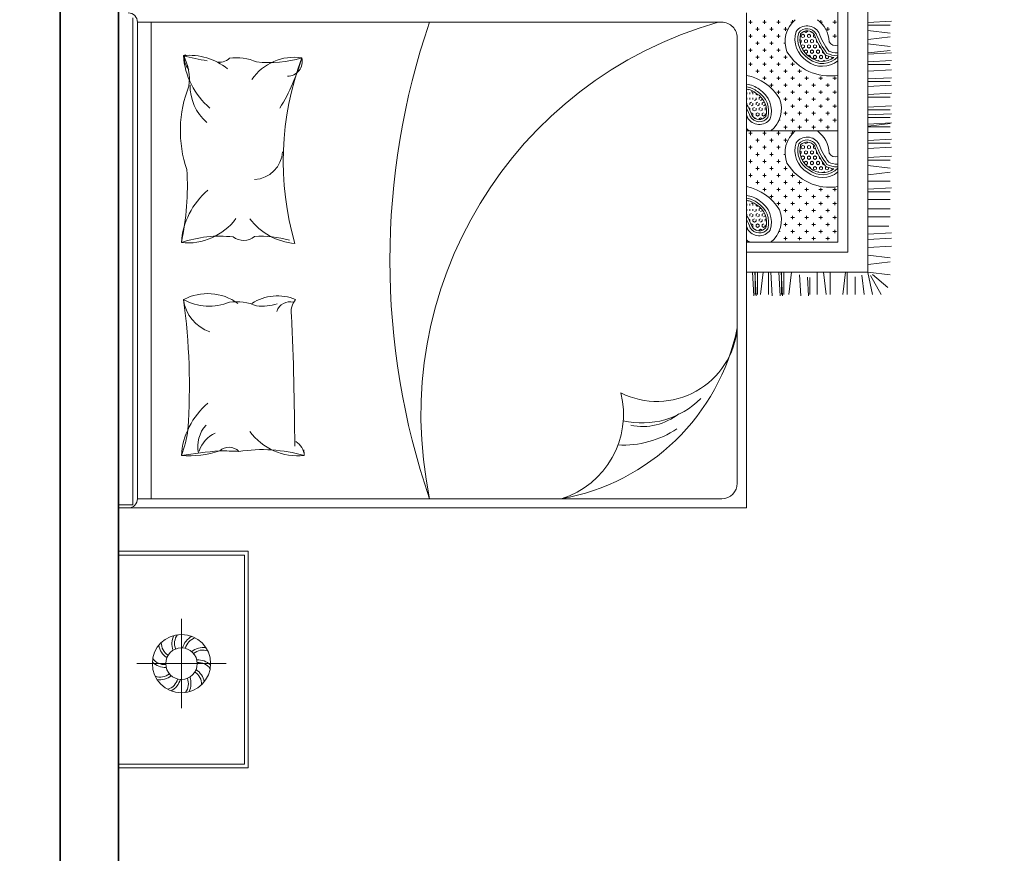
# Model space of a CAD drawing. Units: inches. Extents: x -638 to 186, y -762 to 59.
# Tile 16 of 31: x -168 to -92, y -308 to -243. Entities that reach past the tile are written whole.
import ezdxf

# ---------------------------------------------------------------- set-up
doc = ezdxf.new("R2010")
doc.units = ezdxf.units.IN
for name, color, linetype, lineweight in [('A-ANNO-DIMS', 2, 'Continuous', 18), ('furn', 8, 'Continuous', 13), ('wall', 7, 'Continuous', 35)]:
    doc.layers.add(name, color=color, linetype=linetype, lineweight=lineweight)
doc.styles.get("Standard").update_dxf_attribs({"font": 'arial.ttf'})
doc.dimstyles.new('ISO-25', dxfattribs={"dimtxt": 4, "dimasz": 4, "dimexe": 1.25, "dimexo": 0.625, "dimtad": 0, "dimlunit": 4, "dimtxsty": 'Standard', "dimcen": 2.5, "dimclrt": 256, "dimadec": 0, "dimazin": 0, "dimtfac": 1, "dimtmove": 0, "dimatfit": 3, "dimfxl": 1, "dimfxlon": 1, "dimarcsym": 0})

# ---------------------------------------------------------------- blocks, each defined once
blk = doc.blocks.new('BED-DOUBLE-WITH-NIGHTSTANDS')
for p, q in [((0, 59.951), (78.699, 59.951)), ((0, 49.874), (0, 59.951)), ((0.288, 50.162), (0.288, 59.951)), ((16.508, 59.951), (16.508, 50.162)), ((16.796, 59.951), (16.796, 49.874)), ((20.158, 59.951), (20.158, 11.244)), ((20.398, 58.826), (20.398, 59.951)), ((58.161, 58.826), (20.398, 58.826)), ((8.091, 51.596), (8.091, 58.516)), ((20.878, 58.468), (57.828, 58.468)), ((20.878, 58.468), (20.878, 13.164)), ((57.828, 13.164), (57.828, 58.468)), ((57.828, 57.404), (20.878, 57.404)), ((4.631, 55.056), (11.551, 55.056)), ((16.796, 49.874), (0, 49.874)), ((16.508, 50.162), (0.288, 50.162)), ((22.077, 11.964), (56.628, 11.964)), ((20.158, 11.244), (58.548, 11.244)), ((38.435, 10.789), (36.606, 10.687)), ((38.435, 1.829), (38.435, 11.244)), ((39.99, 3.384), (39.99, 11.244)), ((40.767, 4.161), (40.767, 11.244)), ((41.943, 10.806), (41.98, 10.743)), ((42.116, 10.743), (41.98, 10.743)), ((42.184, 10.861), (42.116, 10.743)), ((42.164, 10.895), (42.184, 10.861)), ((42.388, 10.743), (42.32, 10.625)), ((42.381, 10.99), (42.388, 10.979)), ((42.524, 10.979), (42.388, 10.979)), ((42.524, 10.743), (42.388, 10.743)), ((42.588, 11.09), (42.524, 10.979)), ((42.524, 10.743), (42.592, 10.625)), ((42.728, 10.861), (42.796, 10.743)), ((42.932, 10.979), (42.796, 10.979)), ((42.932, 10.743), (42.796, 10.743)), ((42.932, 11.215), (42.819, 11.215)), ((42.932, 10.979), (43, 10.861)), ((43.34, 11.215), (43.204, 11.215)), ((43.34, 10.979), (43.204, 10.979)), ((43.34, 10.743), (43.204, 10.743)), ((43.748, 11.215), (43.612, 11.215)), ((43.748, 10.979), (43.612, 10.979)), ((43.748, 10.743), (43.612, 10.743)), ((43.816, 10.861), (43.748, 10.743)), ((44.002, 11.184), (43.952, 11.097)), ((45.812, 10.936), (46.084, 10.936)), ((45.948, 10.8), (45.948, 11.072)), ((46.9, 10.936), (47.172, 10.936)), ((47.036, 10.8), (47.036, 11.072)), ((47.989, 10.936), (48.261, 10.936)), ((48.125, 10.8), (48.125, 11.072)), ((49.077, 10.936), (49.349, 10.936)), ((49.213, 10.8), (49.213, 11.072)), ((49.395, 11.244), (49.395, 4.161)), ((50.571, 10.806), (50.607, 10.743)), ((50.743, 10.743), (50.607, 10.743)), ((50.811, 10.861), (50.743, 10.743)), ((50.792, 10.895), (50.811, 10.861)), ((51.015, 10.743), (50.947, 10.625)), ((51.009, 10.99), (51.015, 10.979)), ((51.151, 10.979), (51.015, 10.979)), ((51.151, 10.743), (51.015, 10.743)), ((51.216, 11.09), (51.151, 10.979)), ((51.151, 10.743), (51.219, 10.625)), ((51.355, 10.861), (51.424, 10.743)), ((51.56, 10.979), (51.424, 10.979)), ((51.56, 10.743), (51.424, 10.743)), ((51.56, 11.215), (51.447, 11.215)), ((51.56, 10.979), (51.628, 10.861)), ((51.968, 11.215), (51.832, 11.215)), ((51.968, 10.979), (51.832, 10.979)), ((51.968, 10.743), (51.832, 10.743)), ((52.376, 11.215), (52.24, 11.215)), ((52.376, 10.979), (52.24, 10.979)), ((52.376, 10.743), (52.24, 10.743)), ((52.444, 10.861), (52.376, 10.743)), ((52.63, 11.184), (52.58, 11.097)), ((54.44, 10.936), (54.712, 10.936)), ((54.576, 10.8), (54.576, 11.072)), ((55.528, 10.936), (55.8, 10.936)), ((55.664, 10.8), (55.664, 11.072)), ((56.616, 10.936), (56.888, 10.936)), ((56.752, 10.8), (56.752, 11.072)), ((57.705, 10.936), (57.977, 10.936)), ((57.841, 10.8), (57.841, 11.072)), ((38.435, 10.606), (36.606, 10.504)), ((38.435, 10.585), (36.707, 10.585)), ((38.435, 10.402), (36.707, 10.402)), ((38.435, 9.957), (36.707, 10.161)), ((41.708, 10.272), (41.649, 10.272)), ((41.708, 10.036), (41.685, 10.036)), ((41.708, 10.508), (41.699, 10.508)), ((41.776, 10.625), (41.708, 10.508)), ((41.708, 10.272), (41.776, 10.154)), ((41.776, 10.154), (41.708, 10.036)), ((41.77, 10.636), (41.776, 10.625)), ((41.98, 10.508), (41.912, 10.39)), ((41.912, 10.39), (41.98, 10.272)), ((41.98, 10.036), (41.912, 9.919)), ((42.116, 10.508), (41.98, 10.508)), ((42.116, 10.272), (41.98, 10.272)), ((42.116, 10.036), (41.98, 10.036)), ((42.116, 10.508), (42.184, 10.39)), ((42.184, 10.39), (42.116, 10.272)), ((42.116, 10.036), (42.184, 9.919)), ((42.32, 10.625), (42.388, 10.508)), ((42.32, 10.154), (42.388, 10.036)), ((42.524, 10.508), (42.388, 10.508)), ((42.524, 10.272), (42.388, 10.272)), ((42.524, 10.036), (42.388, 10.036)), ((42.524, 10.272), (42.592, 10.154)), ((42.728, 10.39), (42.796, 10.272)), ((42.932, 10.508), (42.796, 10.508)), ((42.932, 10.272), (42.796, 10.272)), ((42.932, 10.036), (42.796, 10.036)), ((42.932, 10.508), (43, 10.39)), ((42.932, 10.036), (43, 9.919)), ((43.136, 10.625), (43.204, 10.508)), ((43.136, 10.154), (43.204, 10.036)), ((43.34, 10.508), (43.204, 10.508)), ((43.34, 10.272), (43.204, 10.272)), ((43.297, 10.036), (43.204, 10.036)), ((43.34, 10.272), (43.408, 10.154)), ((43.408, 10.154), (43.381, 10.108)), ((43.612, 10.508), (43.544, 10.39)), ((43.703, 10.508), (43.612, 10.508)), ((44.86, 9.711), (44.86, 9.983)), ((45.268, 10.392), (45.54, 10.392)), ((45.404, 10.256), (45.404, 10.528)), ((45.948, 9.711), (45.948, 9.983)), ((46.356, 10.392), (46.628, 10.392)), ((46.492, 10.256), (46.492, 10.528)), ((47.036, 9.711), (47.036, 9.983)), ((47.445, 10.392), (47.717, 10.392)), ((47.581, 10.256), (47.581, 10.528)), ((48.125, 9.711), (48.125, 9.983)), ((48.533, 10.392), (48.805, 10.392)), ((48.669, 10.256), (48.669, 10.528)), ((49.213, 9.711), (49.213, 9.983)), ((50.335, 10.272), (50.277, 10.272)), ((50.335, 10.036), (50.313, 10.036)), ((50.335, 10.508), (50.327, 10.508)), ((50.403, 10.625), (50.335, 10.508)), ((50.335, 10.272), (50.403, 10.154)), ((50.403, 10.154), (50.335, 10.036)), ((50.397, 10.636), (50.403, 10.625)), ((50.607, 10.508), (50.539, 10.39)), ((50.539, 10.39), (50.607, 10.272)), ((50.607, 10.036), (50.539, 9.919)), ((50.743, 10.508), (50.607, 10.508)), ((50.743, 10.272), (50.607, 10.272)), ((50.743, 10.036), (50.607, 10.036)), ((50.743, 10.508), (50.811, 10.39)), ((50.811, 10.39), (50.743, 10.272)), ((50.743, 10.036), (50.811, 9.919)), ((50.947, 10.625), (51.015, 10.508)), ((50.947, 10.154), (51.015, 10.036)), ((51.151, 10.508), (51.015, 10.508)), ((51.151, 10.272), (51.015, 10.272)), ((51.151, 10.036), (51.015, 10.036)), ((51.151, 10.272), (51.219, 10.154)), ((51.355, 10.39), (51.424, 10.272)), ((51.56, 10.508), (51.424, 10.508)), ((51.56, 10.272), (51.424, 10.272)), ((51.56, 10.036), (51.424, 10.036)), ((51.56, 10.508), (51.628, 10.39)), ((51.56, 10.036), (51.628, 9.919)), ((51.764, 10.625), (51.832, 10.508)), ((51.764, 10.154), (51.832, 10.036)), ((51.968, 10.508), (51.832, 10.508)), ((51.968, 10.272), (51.832, 10.272)), ((51.925, 10.036), (51.832, 10.036)), ((51.968, 10.272), (52.036, 10.154)), ((52.036, 10.154), (52.009, 10.108)), ((52.24, 10.508), (52.172, 10.39)), ((52.33, 10.508), (52.24, 10.508)), ((53.487, 9.711), (53.487, 9.983)), ((53.896, 10.392), (54.168, 10.392)), ((54.032, 10.256), (54.032, 10.528)), ((54.576, 9.711), (54.576, 9.983)), ((54.984, 10.392), (55.256, 10.392)), ((55.12, 10.256), (55.12, 10.528)), ((55.664, 9.711), (55.664, 9.983)), ((56.072, 10.392), (56.344, 10.392)), ((56.208, 10.256), (56.208, 10.528)), ((56.752, 9.711), (56.752, 9.983)), ((57.161, 10.392), (57.433, 10.392)), ((57.297, 10.256), (57.297, 10.528)), ((57.841, 9.711), (57.841, 9.983)), ((38.435, 9.347), (36.606, 9.245)), ((38.435, 9.55), (36.707, 9.55)), ((41.912, 9.919), (41.98, 9.801)), ((42.116, 9.801), (41.98, 9.801)), ((42.524, 9.801), (42.388, 9.801)), ((42.524, 9.801), (42.574, 9.713)), ((42.728, 9.919), (42.796, 9.801)), ((42.888, 9.801), (42.796, 9.801)), ((44.18, 9.303), (44.452, 9.303)), ((44.316, 9.167), (44.316, 9.439)), ((44.724, 9.847), (44.996, 9.847)), ((45.268, 9.303), (45.54, 9.303)), ((45.404, 9.167), (45.404, 9.439)), ((45.812, 9.847), (46.084, 9.847)), ((46.356, 9.303), (46.628, 9.303)), ((46.492, 9.167), (46.492, 9.439)), ((46.9, 9.847), (47.172, 9.847)), ((47.445, 9.303), (47.717, 9.303)), ((47.581, 9.167), (47.581, 9.439)), ((47.989, 9.847), (48.261, 9.847)), ((48.533, 9.303), (48.805, 9.303)), ((48.669, 9.167), (48.669, 9.439)), ((49.077, 9.847), (49.349, 9.847)), ((50.539, 9.919), (50.607, 9.801)), ((50.743, 9.801), (50.607, 9.801)), ((51.151, 9.801), (51.015, 9.801)), ((51.151, 9.801), (51.202, 9.713)), ((51.355, 9.919), (51.424, 9.801)), ((51.516, 9.801), (51.424, 9.801)), ((52.807, 9.303), (53.079, 9.303)), ((52.943, 9.167), (52.943, 9.439)), ((53.351, 9.847), (53.623, 9.847)), ((53.896, 9.303), (54.168, 9.303)), ((54.032, 9.167), (54.032, 9.439)), ((54.44, 9.847), (54.712, 9.847)), ((54.984, 9.303), (55.256, 9.303)), ((55.12, 9.167), (55.12, 9.439)), ((55.528, 9.847), (55.8, 9.847)), ((56.072, 9.303), (56.344, 9.303)), ((56.208, 9.167), (56.208, 9.439)), ((56.616, 9.847), (56.888, 9.847)), ((57.161, 9.303), (57.433, 9.303)), ((57.297, 9.167), (57.297, 9.439)), ((57.705, 9.847), (57.977, 9.847)), ((38.435, 8.736), (36.606, 8.634)), ((38.435, 8.553), (36.606, 8.451)), ((38.435, 8.532), (36.707, 8.532)), ((41.459, 8.759), (41.528, 8.759)), ((41.595, 8.623), (41.595, 8.728)), ((43.635, 8.759), (43.907, 8.759)), ((43.771, 8.623), (43.771, 8.895)), ((44.724, 8.759), (44.996, 8.759)), ((44.86, 8.623), (44.86, 8.895)), ((45.812, 8.759), (46.084, 8.759)), ((45.948, 8.623), (45.948, 8.895)), ((46.9, 8.759), (47.172, 8.759)), ((47.036, 8.623), (47.036, 8.895)), ((47.989, 8.759), (48.261, 8.759)), ((48.125, 8.623), (48.125, 8.895)), ((49.077, 8.759), (49.349, 8.759)), ((49.213, 8.623), (49.213, 8.895)), ((50.086, 8.759), (50.155, 8.759)), ((50.222, 8.623), (50.222, 8.728)), ((52.263, 8.759), (52.535, 8.759)), ((52.399, 8.623), (52.399, 8.895)), ((53.351, 8.759), (53.623, 8.759)), ((53.487, 8.623), (53.487, 8.895)), ((54.44, 8.759), (54.712, 8.759)), ((54.576, 8.623), (54.576, 8.895)), ((55.528, 8.759), (55.8, 8.759)), ((55.664, 8.623), (55.664, 8.895)), ((56.616, 8.759), (56.888, 8.759)), ((56.752, 8.623), (56.752, 8.895)), ((57.705, 8.759), (57.977, 8.759)), ((57.841, 8.623), (57.841, 8.895)), ((38.435, 8.349), (36.707, 8.349)), ((38.435, 7.757), (36.707, 7.961)), ((40.914, 8.215), (41.187, 8.215)), ((41.051, 8.079), (41.051, 8.351)), ((41.459, 7.671), (41.731, 7.671)), ((41.595, 7.535), (41.595, 7.807)), ((42.003, 8.215), (42.275, 8.215)), ((42.139, 8.079), (42.139, 8.351)), ((42.547, 7.671), (42.819, 7.671)), ((42.683, 7.535), (42.683, 7.807)), ((43.091, 8.215), (43.363, 8.215)), ((43.227, 8.079), (43.227, 8.351)), ((43.635, 7.671), (43.907, 7.671)), ((43.771, 7.535), (43.771, 7.807)), ((44.18, 8.215), (44.452, 8.215)), ((44.316, 8.079), (44.316, 8.351)), ((44.724, 7.671), (44.996, 7.671)), ((44.86, 7.535), (44.86, 7.807)), ((45.268, 8.215), (45.54, 8.215)), ((45.404, 8.079), (45.404, 8.351)), ((45.812, 7.671), (46.084, 7.671)), ((45.948, 7.535), (45.948, 7.807)), ((46.356, 8.215), (46.628, 8.215)), ((46.492, 8.079), (46.492, 8.351)), ((47.581, 8.253), (47.581, 8.351)), ((48.533, 8.215), (48.805, 8.215)), ((48.669, 8.079), (48.669, 8.351)), ((49.195, 7.671), (49.349, 7.671)), ((49.213, 7.653), (49.213, 7.807)), ((49.542, 8.215), (49.814, 8.215)), ((49.678, 8.079), (49.678, 8.351)), ((50.086, 7.671), (50.358, 7.671)), ((50.222, 7.535), (50.222, 7.807)), ((50.63, 8.215), (50.903, 8.215)), ((50.767, 8.079), (50.767, 8.351)), ((51.175, 7.671), (51.447, 7.671)), ((51.311, 7.535), (51.311, 7.807)), ((51.719, 8.215), (51.991, 8.215)), ((51.855, 8.079), (51.855, 8.351)), ((52.263, 7.671), (52.535, 7.671)), ((52.399, 7.535), (52.399, 7.807)), ((52.807, 8.215), (53.079, 8.215)), ((52.943, 8.079), (52.943, 8.351)), ((53.351, 7.671), (53.623, 7.671)), ((53.487, 7.535), (53.487, 7.807)), ((53.896, 8.215), (54.168, 8.215)), ((54.032, 8.079), (54.032, 8.351)), ((54.44, 7.671), (54.712, 7.671)), ((54.576, 7.535), (54.576, 7.807)), ((54.984, 8.215), (55.256, 8.215)), ((55.12, 8.079), (55.12, 8.351)), ((56.208, 8.253), (56.208, 8.351)), ((57.161, 8.215), (57.433, 8.215)), ((57.297, 8.079), (57.297, 8.351)), ((57.822, 7.671), (57.977, 7.671)), ((57.841, 7.653), (57.841, 7.807)), ((38.233, 7.135), (36.606, 7.044)), ((40.914, 7.127), (41.187, 7.127)), ((41.051, 6.99), (41.051, 7.263)), ((42.003, 7.127), (42.275, 7.127)), ((42.139, 6.99), (42.139, 7.263)), ((43.091, 7.127), (43.363, 7.127)), ((43.227, 6.99), (43.227, 7.263)), ((44.18, 7.127), (44.452, 7.127)), ((44.316, 6.99), (44.316, 7.263)), ((45.268, 7.127), (45.54, 7.127)), ((45.404, 6.99), (45.404, 7.263)), ((47.185, 6.877), (47.239, 6.971)), ((47.253, 6.76), (47.185, 6.877)), ((47.297, 6.995), (47.389, 6.995)), ((47.457, 6.877), (47.389, 6.995)), ((47.389, 6.76), (47.457, 6.877)), ((47.661, 6.995), (47.611, 7.082)), ((47.661, 6.995), (47.797, 6.995)), ((47.797, 6.995), (47.861, 7.105)), ((48.001, 6.877), (48.069, 6.995)), ((48.069, 6.76), (48.001, 6.877)), ((48.069, 6.995), (48.205, 6.995)), ((48.273, 6.877), (48.205, 6.995)), ((48.205, 6.76), (48.273, 6.877)), ((49.542, 7.127), (49.814, 7.127)), ((49.678, 6.99), (49.678, 7.263)), ((50.63, 7.127), (50.903, 7.127)), ((50.767, 6.99), (50.767, 7.263)), ((51.719, 7.127), (51.991, 7.127)), ((51.855, 6.99), (51.855, 7.263)), ((52.807, 7.127), (53.079, 7.127)), ((52.943, 6.99), (52.943, 7.263)), ((53.896, 7.127), (54.168, 7.127)), ((54.032, 6.99), (54.032, 7.263)), ((55.813, 6.877), (55.867, 6.971)), ((55.881, 6.76), (55.813, 6.877)), ((55.924, 6.995), (56.017, 6.995)), ((56.085, 6.877), (56.017, 6.995)), ((56.017, 6.76), (56.085, 6.877)), ((56.289, 6.995), (56.238, 7.082)), ((56.289, 6.995), (56.425, 6.995)), ((56.425, 6.995), (56.488, 7.105)), ((56.629, 6.877), (56.697, 6.995)), ((56.697, 6.76), (56.629, 6.877)), ((56.697, 6.995), (56.833, 6.995)), ((56.901, 6.877), (56.833, 6.995)), ((56.833, 6.76), (56.901, 6.877)), ((38.06, 6.514), (36.606, 6.433)), ((38.024, 6.332), (36.707, 6.332)), ((41.051, 5.902), (41.051, 6.174)), ((41.459, 6.582), (41.731, 6.582)), ((41.595, 6.446), (41.595, 6.718)), ((42.139, 5.902), (42.139, 6.174)), ((42.547, 6.582), (42.819, 6.582)), ((42.683, 6.446), (42.683, 6.718)), ((43.227, 5.902), (43.227, 6.174)), ((43.635, 6.582), (43.907, 6.582)), ((43.771, 6.446), (43.771, 6.718)), ((44.316, 5.902), (44.316, 6.174)), ((44.724, 6.582), (44.996, 6.582)), ((44.86, 6.446), (44.86, 6.718)), ((46.482, 6.288), (46.573, 6.288)), ((46.573, 6.288), (46.641, 6.406)), ((46.641, 6.406), (46.605, 6.469)), ((46.777, 6.642), (46.803, 6.688)), ((46.845, 6.524), (46.777, 6.642)), ((46.777, 6.17), (46.845, 6.288)), ((46.845, 6.053), (46.777, 6.17)), ((46.845, 6.524), (46.981, 6.524)), ((46.845, 6.288), (46.981, 6.288)), ((46.888, 6.76), (46.981, 6.76)), ((47.049, 6.642), (46.981, 6.76)), ((46.981, 6.524), (47.049, 6.642)), ((47.049, 6.17), (46.981, 6.288)), ((46.981, 6.053), (47.049, 6.17)), ((47.185, 6.406), (47.253, 6.524)), ((47.253, 6.288), (47.185, 6.406)), ((47.253, 6.76), (47.389, 6.76)), ((47.253, 6.524), (47.389, 6.524)), ((47.253, 6.288), (47.389, 6.288)), ((47.457, 6.406), (47.389, 6.524)), ((47.389, 6.288), (47.457, 6.406)), ((47.593, 6.642), (47.661, 6.76)), ((47.661, 6.524), (47.593, 6.642)), ((47.593, 6.17), (47.661, 6.288)), ((47.661, 6.053), (47.593, 6.17)), ((47.661, 6.76), (47.797, 6.76)), ((47.661, 6.524), (47.797, 6.524)), ((47.661, 6.288), (47.797, 6.288)), ((47.865, 6.642), (47.797, 6.76)), ((47.797, 6.524), (47.865, 6.642)), ((47.865, 6.17), (47.797, 6.288)), ((47.797, 6.053), (47.865, 6.17)), ((48.001, 6.406), (48.069, 6.524)), ((48.069, 6.288), (48.001, 6.406)), ((48.069, 6.76), (48.205, 6.76)), ((48.069, 6.524), (48.205, 6.524)), ((48.069, 6.288), (48.205, 6.288)), ((48.273, 6.406), (48.205, 6.524)), ((48.205, 6.288), (48.273, 6.406)), ((48.409, 6.642), (48.477, 6.76)), ((48.477, 6.524), (48.409, 6.642)), ((48.409, 6.17), (48.477, 6.288)), ((48.415, 6.16), (48.409, 6.17)), ((48.477, 6.76), (48.5, 6.76)), ((48.477, 6.524), (48.536, 6.524)), ((48.477, 6.288), (48.486, 6.288)), ((49.678, 5.902), (49.678, 6.174)), ((50.086, 6.582), (50.358, 6.582)), ((50.222, 6.446), (50.222, 6.718)), ((50.767, 5.902), (50.767, 6.174)), ((51.175, 6.582), (51.447, 6.582)), ((51.311, 6.446), (51.311, 6.718)), ((51.855, 5.902), (51.855, 6.174)), ((52.263, 6.582), (52.535, 6.582)), ((52.399, 6.446), (52.399, 6.718)), ((52.943, 5.902), (52.943, 6.174)), ((53.351, 6.582), (53.623, 6.582)), ((53.487, 6.446), (53.487, 6.718)), ((55.11, 6.288), (55.201, 6.288)), ((55.201, 6.288), (55.269, 6.406)), ((55.269, 6.406), (55.232, 6.469)), ((55.405, 6.642), (55.431, 6.688)), ((55.473, 6.524), (55.405, 6.642)), ((55.405, 6.17), (55.473, 6.288)), ((55.473, 6.053), (55.405, 6.17)), ((55.473, 6.524), (55.609, 6.524)), ((55.473, 6.288), (55.609, 6.288)), ((55.515, 6.76), (55.609, 6.76)), ((55.677, 6.642), (55.609, 6.76)), ((55.609, 6.524), (55.677, 6.642)), ((55.677, 6.17), (55.609, 6.288)), ((55.609, 6.053), (55.677, 6.17)), ((55.813, 6.406), (55.881, 6.524)), ((55.881, 6.288), (55.813, 6.406)), ((55.881, 6.76), (56.017, 6.76)), ((55.881, 6.524), (56.017, 6.524)), ((55.881, 6.288), (56.017, 6.288)), ((56.085, 6.406), (56.017, 6.524)), ((56.017, 6.288), (56.085, 6.406)), ((56.221, 6.642), (56.289, 6.76)), ((56.289, 6.524), (56.221, 6.642)), ((56.221, 6.17), (56.289, 6.288)), ((56.289, 6.053), (56.221, 6.17)), ((56.289, 6.76), (56.425, 6.76)), ((56.289, 6.524), (56.425, 6.524)), ((56.289, 6.288), (56.425, 6.288)), ((56.493, 6.642), (56.425, 6.76)), ((56.425, 6.524), (56.493, 6.642)), ((56.493, 6.17), (56.425, 6.288)), ((56.425, 6.053), (56.493, 6.17)), ((56.629, 6.406), (56.697, 6.524)), ((56.697, 6.288), (56.629, 6.406)), ((56.697, 6.76), (56.833, 6.76)), ((56.697, 6.524), (56.833, 6.524)), ((56.697, 6.288), (56.833, 6.288)), ((56.901, 6.406), (56.833, 6.524)), ((56.833, 6.288), (56.901, 6.406)), ((57.037, 6.642), (57.105, 6.76)), ((57.105, 6.524), (57.037, 6.642)), ((57.037, 6.17), (57.105, 6.288)), ((57.043, 6.16), (57.037, 6.17)), ((57.105, 6.76), (57.128, 6.76)), ((57.105, 6.524), (57.164, 6.524)), ((57.105, 6.288), (57.113, 6.288)), ((38.435, 5.764), (36.71, 5.764)), ((40.914, 6.038), (41.187, 6.038)), ((41.459, 5.494), (41.731, 5.494)), ((41.595, 5.358), (41.595, 5.63)), ((42.003, 6.038), (42.275, 6.038)), ((42.547, 5.494), (42.819, 5.494)), ((42.683, 5.358), (42.683, 5.63)), ((43.091, 6.038), (43.363, 6.038)), ((43.635, 5.494), (43.907, 5.494)), ((43.771, 5.358), (43.771, 5.63)), ((44.18, 6.038), (44.452, 6.038)), ((44.724, 5.494), (44.996, 5.494)), ((44.86, 5.358), (44.86, 5.63)), ((46.162, 5.346), (46.165, 5.346)), ((46.233, 5.228), (46.165, 5.346)), ((46.183, 5.612), (46.233, 5.699)), ((46.233, 5.699), (46.21, 5.739)), ((46.369, 5.935), (46.437, 6.053)), ((46.437, 5.817), (46.369, 5.935)), ((46.369, 5.464), (46.437, 5.581)), ((46.437, 5.346), (46.369, 5.464)), ((46.437, 6.053), (46.573, 6.053)), ((46.437, 5.817), (46.573, 5.817)), ((46.437, 5.581), (46.573, 5.581)), ((46.437, 5.346), (46.573, 5.346)), ((46.641, 5.935), (46.573, 6.053)), ((46.573, 5.817), (46.641, 5.935)), ((46.641, 5.464), (46.573, 5.581)), ((46.573, 5.346), (46.641, 5.464)), ((46.777, 5.699), (46.845, 5.817)), ((46.845, 5.581), (46.777, 5.699)), ((46.777, 5.228), (46.845, 5.346)), ((46.845, 6.053), (46.981, 6.053)), ((46.845, 5.817), (46.981, 5.817)), ((46.845, 5.581), (46.981, 5.581)), ((46.845, 5.346), (46.981, 5.346)), ((47.049, 5.699), (46.981, 5.817)), ((46.981, 5.581), (47.049, 5.699)), ((46.982, 5.344), (46.981, 5.346)), ((47.185, 5.935), (47.253, 6.053)), ((47.253, 5.817), (47.185, 5.935)), ((47.195, 5.481), (47.253, 5.581)), ((47.253, 6.053), (47.389, 6.053)), ((47.253, 5.817), (47.389, 5.817)), ((47.253, 5.581), (47.365, 5.581)), ((47.457, 5.935), (47.389, 6.053)), ((47.389, 5.817), (47.457, 5.935)), ((47.597, 5.706), (47.661, 5.817)), ((47.661, 6.053), (47.797, 6.053)), ((47.661, 5.817), (47.797, 5.817)), ((47.804, 5.806), (47.797, 5.817)), ((48.001, 5.935), (48.069, 6.053)), ((48.021, 5.901), (48.001, 5.935)), ((48.069, 6.053), (48.205, 6.053)), ((48.242, 5.99), (48.205, 6.053)), ((49.542, 6.038), (49.814, 6.038)), ((50.086, 5.494), (50.358, 5.494)), ((50.222, 5.358), (50.222, 5.63)), ((50.63, 6.038), (50.903, 6.038)), ((51.175, 5.494), (51.447, 5.494)), ((51.311, 5.358), (51.311, 5.63)), ((51.719, 6.038), (51.991, 6.038)), ((52.263, 5.494), (52.535, 5.494)), ((52.399, 5.358), (52.399, 5.63)), ((52.807, 6.038), (53.079, 6.038)), ((53.351, 5.494), (53.623, 5.494)), ((53.487, 5.358), (53.487, 5.63)), ((54.789, 5.346), (54.792, 5.346)), ((54.86, 5.228), (54.792, 5.346)), ((54.81, 5.612), (54.86, 5.699)), ((54.86, 5.699), (54.837, 5.739)), ((54.996, 5.935), (55.064, 6.053)), ((55.064, 5.817), (54.996, 5.935)), ((54.996, 5.464), (55.064, 5.581)), ((55.064, 5.346), (54.996, 5.464)), ((55.064, 6.053), (55.201, 6.053)), ((55.064, 5.817), (55.201, 5.817)), ((55.064, 5.581), (55.201, 5.581)), ((55.064, 5.346), (55.201, 5.346)), ((55.269, 5.935), (55.201, 6.053)), ((55.201, 5.817), (55.269, 5.935)), ((55.269, 5.464), (55.201, 5.581)), ((55.201, 5.346), (55.269, 5.464)), ((55.405, 5.699), (55.473, 5.817)), ((55.473, 5.581), (55.405, 5.699)), ((55.405, 5.228), (55.473, 5.346)), ((55.473, 6.053), (55.609, 6.053)), ((55.473, 5.817), (55.609, 5.817)), ((55.473, 5.581), (55.609, 5.581)), ((55.473, 5.346), (55.609, 5.346)), ((55.677, 5.699), (55.609, 5.817)), ((55.609, 5.581), (55.677, 5.699)), ((55.609, 5.344), (55.609, 5.346)), ((55.813, 5.935), (55.881, 6.053)), ((55.881, 5.817), (55.813, 5.935)), ((55.823, 5.481), (55.881, 5.581)), ((55.881, 6.053), (56.017, 6.053)), ((55.881, 5.817), (56.017, 5.817)), ((55.881, 5.581), (55.993, 5.581)), ((56.085, 5.935), (56.017, 6.053)), ((56.017, 5.817), (56.085, 5.935)), ((56.225, 5.706), (56.289, 5.817)), ((56.289, 6.053), (56.425, 6.053)), ((56.289, 5.817), (56.425, 5.817)), ((56.431, 5.806), (56.425, 5.817)), ((56.629, 5.935), (56.697, 6.053)), ((56.649, 5.901), (56.629, 5.935)), ((56.697, 6.053), (56.833, 6.053)), ((56.869, 5.99), (56.833, 6.053)), ((57.803, 5.494), (57.977, 5.494)), ((57.841, 5.358), (57.841, 5.533)), ((38.435, 5.274), (36.707, 5.069)), ((38.435, 4.769), (36.71, 4.769)), ((40.914, 4.95), (41.187, 4.95)), ((41.051, 4.814), (41.051, 5.086)), ((42.003, 4.95), (42.275, 4.95)), ((42.139, 4.814), (42.139, 5.086)), ((43.091, 4.95), (43.363, 4.95)), ((43.227, 4.814), (43.227, 5.086)), ((44.18, 4.95), (44.452, 4.95)), ((44.316, 4.814), (44.316, 5.086)), ((46.179, 5.135), (46.233, 5.228)), ((46.369, 4.992), (46.437, 5.11)), ((46.437, 4.874), (46.369, 4.992)), ((46.393, 4.563), (46.437, 4.639)), ((46.437, 5.11), (46.573, 5.11)), ((46.437, 4.874), (46.559, 4.874)), ((46.437, 4.639), (46.493, 4.639)), ((46.619, 5.03), (46.573, 5.11)), ((46.788, 5.209), (46.777, 5.228)), ((49.542, 4.95), (49.814, 4.95)), ((49.678, 4.814), (49.678, 5.086)), ((50.63, 4.95), (50.903, 4.95)), ((50.767, 4.814), (50.767, 5.086)), ((51.719, 4.95), (51.991, 4.95)), ((51.855, 4.814), (51.855, 5.086)), ((52.807, 4.95), (53.079, 4.95)), ((52.943, 4.814), (52.943, 5.086)), ((54.807, 5.135), (54.86, 5.228)), ((54.996, 4.992), (55.064, 5.11)), ((55.064, 4.874), (54.996, 4.992)), ((55.021, 4.563), (55.064, 4.639)), ((55.064, 5.11), (55.201, 5.11)), ((55.064, 4.874), (55.187, 4.874)), ((55.064, 4.639), (55.12, 4.639)), ((55.247, 5.03), (55.201, 5.11)), ((55.416, 5.209), (55.405, 5.228)), ((57.161, 4.95), (57.433, 4.95)), ((57.297, 4.814), (57.297, 5.086)), ((66.65, 4.161), (40.767, 4.161)), ((41.459, 4.406), (41.731, 4.406)), ((41.595, 4.27), (41.595, 4.542)), ((42.547, 4.406), (42.819, 4.406)), ((42.683, 4.27), (42.683, 4.542)), ((43.635, 4.406), (43.907, 4.406)), ((43.771, 4.27), (43.771, 4.542)), ((44.724, 4.406), (44.996, 4.406)), ((44.86, 4.27), (44.86, 4.542)), ((50.086, 4.406), (50.358, 4.406)), ((50.222, 4.27), (50.222, 4.542)), ((51.175, 4.406), (51.447, 4.406)), ((51.311, 4.27), (51.311, 4.542)), ((52.263, 4.406), (52.535, 4.406)), ((52.399, 4.27), (52.399, 4.542)), ((53.351, 4.406), (53.623, 4.406)), ((53.487, 4.27), (53.487, 4.542)), ((56.616, 4.406), (56.888, 4.406)), ((56.752, 4.27), (56.752, 4.542)), ((57.705, 4.406), (57.977, 4.406)), ((57.841, 4.27), (57.841, 4.542)), ((38.435, 3.565), (36.707, 3.769)), ((38.435, 3.446), (36.71, 3.446)), ((67.427, 3.384), (39.99, 3.384)), ((38.221, 2.295), (36.707, 2.115)), ((38.086, 2.81), (36.71, 2.81)), ((38.185, 1.631), (36.707, 0.792)), ((38.421, 1.829), (36.71, 1.486)), ((38.435, 1.829), (38.231, 0.102)), ((68.982, 1.829), (38.435, 1.829)), ((39.046, 1.815), (39.249, 0.102)), ((39.759, 1.829), (39.555, 0.102)), ((40.369, 1.829), (40.471, 0)), ((40.98, 1.829), (41.082, 0)), ((41.388, 1.829), (41.49, 0)), ((41.999, 1.829), (41.999, 0.203)), ((42.744, 1.829), (42.744, 0.102)), ((43.355, 1.829), (43.355, 0.102)), ((44.068, 1.829), (44.068, 0.102)), ((44.679, 1.829), (44.679, 0.102)), ((44.882, 1.829), (44.984, 0)), ((45.511, 1.815), (45.511, 0.105)), ((46.002, 1.815), (46.206, 0.102)), ((46.715, 1.829), (46.512, 0.102)), ((47.122, 1.829), (47.122, 0.102)), ((47.326, 1.829), (47.428, 0)), ((48.039, 1.829), (48.141, 0)), ((48.446, 1.829), (48.446, 0.102)), ((48.65, 1.829), (48.752, 0)), ((49.279, 1.815), (49.279, 0.105)), ((49.717, 1.829), (49.717, 0.102)), ((49.77, 1.815), (49.973, 0.102)), ((49.92, 1.829), (50.022, 0)), ((50.429, 1.829), (50.429, 0.102)), ((50.633, 1.829), (50.735, 0)), ((51.04, 1.829), (51.04, 0.102)), ((51.244, 1.829), (51.346, 0)), ((52.025, 1.829), (52.025, 0.102)), ((52.229, 1.829), (52.331, 0)), ((52.84, 1.829), (52.942, 0)), ((53.221, 1.829), (53.221, 0.102)), ((53.424, 1.829), (53.526, 0)), ((54.035, 1.829), (54.137, 0)), ((54.544, 1.829), (54.544, 0.102)), ((54.748, 1.829), (54.85, 0)), ((55.359, 1.829), (55.461, 0)), ((55.442, 1.815), (55.646, 0.102)), ((56.155, 1.829), (55.951, 0.102)), ((56.479, 1.815), (56.683, 0.102)), ((57.192, 1.829), (56.988, 0.102)), ((57.599, 1.829), (57.599, 0.102)), ((57.803, 1.829), (57.905, 0)), ((38.274, 1.47), (37.248, 0.275))]:
    blk.add_line(p, q)
for radius in [2.26, 1.225]:
    blk.add_circle((8.091, 55.056), radius)
for centre, radius, start, end in [((20.878, 59.188), 0.72, 180, 270), ((57.828, 59.188), 0.72, 270, 0), ((9.248, 56.308), 1.452, 136.17003, 182.48975), ((9.115, 56.366), 1.108, 124.30017, 184.53802), ((8.292, 56.749), 1.452, 172.17003, 218.48975), ((8.15, 56.718), 1.108, 160.30017, 220.53802), ((9.763, 55.389), 1.452, 100.17003, 146.48975), ((9.69, 55.514), 1.108, 88.30017, 148.53802), ((7.258, 56.544), 1.452, 208.17003, 254.48975), ((7.162, 56.435), 1.108, 196.30017, 256.53802), ((9.64, 54.343), 1.452, 64.17003, 110.48975), ((9.653, 54.487), 1.108, 52.30017, 112.53802), ((31.6, 54.462), 7.401, 175.30484, 198.69419), ((-14.535, 48.797), 39.263, 4.80985, 9.18918), ((26.929, 61.603), 7.073, 247.51785, 264.26696), ((23.812, 49.204), 5.878, 40.4189, 85.9871), ((45.371, 54.589), 4.662, 174.11002, 233.4289), ((45.094, 75.141), 20.542, 257.74383, 273.62843), ((40.322, 49.204), 5.878, 40.4189, 85.9871), ((32.161, 52.085), 9.076, 353.49469, 19.18669), ((49.42, 45.842), 9.304, 68.20259, 108.9817), ((6.529, 55.625), 1.108, 232.30017, 292.53802), ((6.543, 55.77), 1.452, 244.17003, 290.48975), ((7.891, 53.363), 1.452, 352.17003, 38.48975), ((9.021, 53.678), 1.108, 16.30017, 76.53802), ((8.925, 53.569), 1.452, 28.17003, 74.48975), ((29.668, 101.849), 47.41, 265.83211, 278.05982), ((36.728, 51.85), 3.086, 97.70317, 160.97754), ((40.051, 52.903), 4.24, 151.77364, 201.69827), ((32.811, 53.035), 3.973, 323.73888, 28.12687), ((52.894, 50.642), 3.752, 88.95772, 139.05179), ((55.647, 49.045), 5.878, 94.0129, 139.5811), ((53.423, 58.191), 3.75, 261.59582, 298.90918), ((54.987, 53.651), 1.175, 72.9226, 134.40089), ((50.598, 54.43), 4.662, 320.94042, 5.88999), ((67.137, 51.406), 12.406, 163.60457, 172.3273), ((6.493, 54.599), 1.108, 268.30017, 328.53802), ((6.419, 54.723), 1.452, 280.17003, 326.48975), ((7.067, 53.747), 1.108, 304.30017, 4.53802), ((6.934, 53.804), 1.452, 316.17003, 2.48975), ((8.033, 53.395), 1.108, 340.30017, 40.53802), ((24.909, 51.33), 2.472, 47.45091, 101.77931), ((23.874, 51.513), 2.284, 23.87557, 72.13833), ((23.796, 51.371), 1.071, 314.4736, 42.17134), ((-32.064, 53.187), 56.669, 357.39054, 358.88764), ((55.833, 52.089), 1.101, 165.35061, 223.26844), ((32.112, 50.806), 4.034, 337.01696, 7.53676), ((51.033, 50.806), 4.034, 337.01696, 7.53676), ((12.792, 48.807), 11.891, 344.0243, 8.70709), ((42.214, 50.25), 1.313, 142.08329, 220.902), ((28.862, 46.013), 4.662, 126.5711, 185.88998), ((45.546, 45.855), 4.894, 127.11975, 175.09005), ((40.21, 48.864), 4.4, 175.22328, 196.23004), ((32.952, 47.606), 3.653, 337.44667, 33.04781), ((33.322, 48.899), 7.916, 343.79543, 3.55541), ((47.91, 49.493), 2.28, 182.63002, 266.88402), ((51.147, 46.324), 3.96, 351.26213, 55.75721), ((63.68, 48.265), 8.986, 173.82958, 196.4356), ((35.105, 46.659), 1.047, 343.35206, 73.29947), ((59.196, 60.444), 15.291, 238.34989, 254.31375), ((47.026, 24.056), 23.109, 69.65065, 105.96307), ((54.788, 46.836), 1.147, 179.77267, 283.80184), ((24.141, 46.898), 1.366, 273.47085, 328.54118), ((24.019, 282.807), 236.536, 270.22759, 272.68343), ((35.378, 45.11), 1.447, 49.09906, 101.37023), ((23.812, 51.397), 5.878, 274.0129, 278.34166), ((39.353, -18.016), 56.914, 71.05766, 108.94234), ((27.358, 4.824), 31.662, 15.77081, 101.80991), ((37.529, 28.521), 16.903, 189.91062, 258.38345), ((27.435, 27.646), 6.865, 197.236, 283.86348), ((32.674, 20.841), 7.64, 177.22468, 213.41029), ((33.202, 19.362), 6.454, 167.11557, 225.10482), ((34.672, 18.19), 6.25, 153.48354, 264.97652), ((30.992, 19.307), 4.516, 168.35906, 218.53383), ((22.077, 13.164), 1.2, 180, 270), ((56.628, 13.164), 1.2, 270, 360), ((42.601, 9.717), 2.246, 137.14315, 144.73933), ((42.315, 10.253), 1.047, 120.34402, 234.01917), ((42.315, 10.253), 0.829, 121.62322, 231.69571), ((42.315, 10.253), 0.666, 122.94981, 229.099), ((39.887, 16.395), 5.571, 289.92189, 292.41183), ((39.887, 16.395), 5.789, 290.13177, 297.16349), ((39.887, 16.395), 5.952, 290.29972, 300.08235), ((41.275, 12.01), 3.88, 301.11254, 348.61386), ((42.526, 11.434), 1.497, 320.65411, 352.72896), ((42.526, 11.434), 1.66, 321.11073, 353.44716), ((42.526, 11.434), 1.878, 321.59726, 354.2094), ((51.228, 9.717), 2.246, 137.14315, 144.73933), ((50.942, 10.253), 1.047, 120.34402, 234.01917), ((50.942, 10.253), 0.829, 121.62322, 231.69571), ((50.942, 10.253), 0.666, 122.94981, 229.099), ((48.515, 16.395), 5.571, 289.92189, 292.41183), ((48.515, 16.395), 5.789, 290.13177, 297.16349), ((48.515, 16.395), 5.952, 290.29972, 300.08235), ((49.903, 12.01), 3.88, 301.11254, 348.61386), ((51.154, 11.434), 1.497, 320.65411, 352.72896), ((51.154, 11.434), 1.66, 321.11073, 353.44716), ((51.154, 11.434), 1.878, 321.59726, 354.2094), ((42.307, 11.282), 1.972, 252.05502, 329.01896), ((42.307, 11.282), 1.754, 253.21886, 329.48085), ((42.307, 11.282), 1.591, 254.37381, 329.91174), ((50.935, 11.282), 1.972, 252.05502, 329.01896), ((50.935, 11.282), 1.754, 253.21886, 329.48085), ((50.935, 11.282), 1.591, 254.37381, 329.91174), ((42.485, 10.742), 2.202, 218.7027, 291.15831), ((51.113, 10.742), 2.202, 218.7027, 291.15831), ((48.91, 4.786), 3.88, 121.11254, 189.2666), ((47.7, 6.054), 2.202, 39.66533, 111.15831), ((57.538, 4.786), 3.88, 121.11254, 189.2666), ((56.328, 6.054), 2.202, 39.66533, 111.15831), ((47.878, 5.514), 1.972, 72.05502, 149.01896), ((47.878, 5.514), 1.754, 73.21886, 149.48085), ((47.878, 5.514), 1.591, 74.37381, 149.91174), ((47.87, 6.543), 0.666, 302.94981, 49.099), ((47.87, 6.543), 0.829, 301.62322, 51.69571), ((47.87, 6.543), 1.047, 300.34402, 54.01917), ((56.505, 5.514), 1.972, 72.05502, 149.01896), ((56.505, 5.514), 1.754, 73.21886, 149.48085), ((56.505, 5.514), 1.591, 74.37381, 149.91174), ((56.498, 6.543), 0.666, 302.94981, 49.099), ((56.498, 6.543), 0.829, 301.62322, 51.69571), ((56.498, 6.543), 1.047, 300.34402, 54.01917), ((47.659, 5.362), 1.878, 141.59726, 219.76108), ((47.659, 5.362), 1.66, 141.11073, 226.3387), ((47.659, 5.362), 1.497, 140.65411, 216.833), ((56.286, 5.362), 1.878, 141.59726, 219.76108), ((56.286, 5.362), 1.66, 141.11073, 226.3387), ((56.286, 5.362), 1.497, 140.65411, 216.833), ((50.298, 0.401), 5.952, 110.29972, 127.73852), ((50.298, 0.401), 5.789, 110.13177, 127.34596), ((50.298, 0.401), 5.571, 109.92189, 126.76774), ((47.584, 7.079), 2.246, 272.46753, 323.71933), ((58.925, 0.401), 5.952, 110.29972, 127.73852), ((58.925, 0.401), 5.789, 110.13177, 127.34596), ((58.925, 0.401), 5.571, 109.92189, 126.76774), ((56.212, 7.079), 2.246, 272.46753, 323.71933), ((48.704, 4.14), 2.268, 154.70595, 171.7535), ((48.704, 4.14), 2.104, 155.76091, 178.03728), ((48.704, 4.14), 1.887, 157.40908, 178.03728), ((47.926, 4.355), 0.54, 117.00881, 201.04089), ((57.332, 4.14), 2.268, 154.70595, 171.7535), ((57.332, 4.14), 2.104, 155.76091, 178.03728), ((57.332, 4.14), 1.887, 157.40908, 178.03728), ((56.554, 4.355), 0.54, 117.00881, 201.04089)]:
    blk.add_arc(centre, radius, start, end)
blk = doc.blocks.new('*D37')
at = {"layer": 'A-ANNO-DIMS', "color": 0, "lineweight": -2, "transparency": 16777216}
for p, q in [((182.663, -232.533), (184.913, -232.533)), ((183.663, -236.533), (183.663, -250.511)), ((183.663, -276.533), (183.663, -262.555)), ((182.663, -280.533), (184.913, -280.533))]:
    blk.add_line(p, q, dxfattribs=at)
at = {"layer": 'A-ANNO-DIMS', "color": 0, "lineweight": 30, "transparency": 16777216}
for points in [[(182.997, -236.533), (184.33, -236.533), (183.663, -232.533)], [(182.997, -276.533), (184.33, -276.533), (183.663, -280.533)]]:
    blk.add_solid(points, dxfattribs=at)
at = {"layer": 'Defpoints', "color": 0, "lineweight": 30, "transparency": 16777216}
for p in [(-404.526, -232.533), (-404.526, -280.533), (183.663, -280.533)]:
    blk.add_point(p, dxfattribs=at)
at = {"layer": 'A-ANNO-DIMS', "transparency": 16777216, "insert": (183.663, -256.533), "char_height": 4, "attachment_point": 5, "rotation": 90}
blk.add_mtext('4\'-0"', dxfattribs=at)
blk = doc.blocks.new('*D38')
at = {"layer": 'A-ANNO-DIMS', "color": 0, "lineweight": -2, "transparency": 16777216}
for p, q in [((182.663, -280.533), (184.913, -280.533)), ((183.663, -284.533), (183.663, -371.726)), ((183.663, -473.533), (183.663, -386.34)), ((182.663, -477.533), (184.913, -477.533))]:
    blk.add_line(p, q, dxfattribs=at)
at = {"layer": 'A-ANNO-DIMS', "color": 0, "lineweight": 30, "transparency": 16777216}
for points in [[(182.997, -284.533), (184.33, -284.533), (183.663, -280.533)], [(182.997, -473.533), (184.33, -473.533), (183.663, -477.533)]]:
    blk.add_solid(points, dxfattribs=at)
at = {"layer": 'Defpoints', "color": 0, "lineweight": 30, "transparency": 16777216}
for p in [(-404.526, -280.533), (-404.526, -477.533), (183.663, -477.533)]:
    blk.add_point(p, dxfattribs=at)
at = {"layer": 'A-ANNO-DIMS', "transparency": 16777216, "insert": (183.663, -379.033), "char_height": 4, "attachment_point": 5, "rotation": 90}
blk.add_mtext('16\'-5"', dxfattribs=at)
blk = doc.blocks.new('*D56')
at = {"layer": 'A-ANNO-DIMS', "color": 0, "lineweight": -2, "transparency": 16777216}
for p, q in [((-165.026, 52.017), (-165.026, 54.267)), ((-100.526, 52.017), (-100.526, 54.267)), ((-161.026, 53.017), (-143.378, 53.017)), ((-104.526, 53.017), (-122.174, 53.017))]:
    blk.add_line(p, q, dxfattribs=at)
at = {"layer": 'A-ANNO-DIMS', "color": 0, "lineweight": 30, "transparency": 16777216}
for points in [[(-161.026, 53.684), (-161.026, 52.35), (-165.026, 53.017)], [(-104.526, 53.684), (-104.526, 52.35), (-100.526, 53.017)]]:
    blk.add_solid(points, dxfattribs=at)
at = {"layer": 'Defpoints', "color": 0, "lineweight": 30, "transparency": 16777216}
for p in [(-100.526, 53.017), (-165.026, -408.033), (-100.526, -408.033)]:
    blk.add_point(p, dxfattribs=at)
at = {"layer": 'A-ANNO-DIMS', "transparency": 16777216, "insert": (-132.776, 53.017), "char_height": 4, "attachment_point": 5}
blk.add_mtext('5\'-4 1/2"', dxfattribs=at)

msp = doc.modelspace()

# ---------------------------------------------------------------- linework, layer by layer
at = {"layer": 'wall'}
for p, q in [((-165.026, -197.592), (-165.026, -354.033)), ((-160.526, -205.533), (-160.526, -349.533))]:
    msp.add_line(p, q, dxfattribs=at)

# ---------------------------------------------------------------- block references
at = {"layer": 'furn', "rotation": 90.00000000000006}
msp.add_blockref('BED-DOUBLE-WITH-NIGHTSTANDS', (-100.575, -301.287), dxfattribs=at)

# ---------------------------------------------------------------- dimensions: what is measured, and where the dimension line sits
at = {"layer": 'A-ANNO-DIMS'}
dim = msp.add_linear_dim(base=(-100.526, 53.017), p1=(-165.026, -408.033), p2=(-100.526, -408.033), dimstyle='ISO-25', override={"dimdec": 1, "dimlfac": 1, "dimrnd": 0, "dimzin": 1, "dimdsep": 46, "dimlunit": 4, "dimfrac": 2}, dxfattribs=at)
dim.commit()
dim.dimension.update_dxf_attribs({"geometry": '*D56', "text_midpoint": (-132.776, 53.017)})
for base, p1, p2, picture, middle in [((183.663, -280.533), (-404.526, -232.533), (-404.526, -280.533), '*D37', (183.663, -256.533)), ((183.663, -477.533), (-404.526, -280.533), (-404.526, -477.533), '*D38', (183.663, -379.033))]:
    dim = msp.add_linear_dim(base=base, p1=p1, p2=p2, angle=90, dimstyle='ISO-25', override={"dimdec": 1, "dimlfac": 1, "dimrnd": 0, "dimzin": 1, "dimdsep": 46, "dimlunit": 4, "dimfrac": 2}, dxfattribs=at)
    dim.commit()
    dim.dimension.update_dxf_attribs({"geometry": picture, "text_midpoint": middle})

doc.saveas('drawing.dxf')
